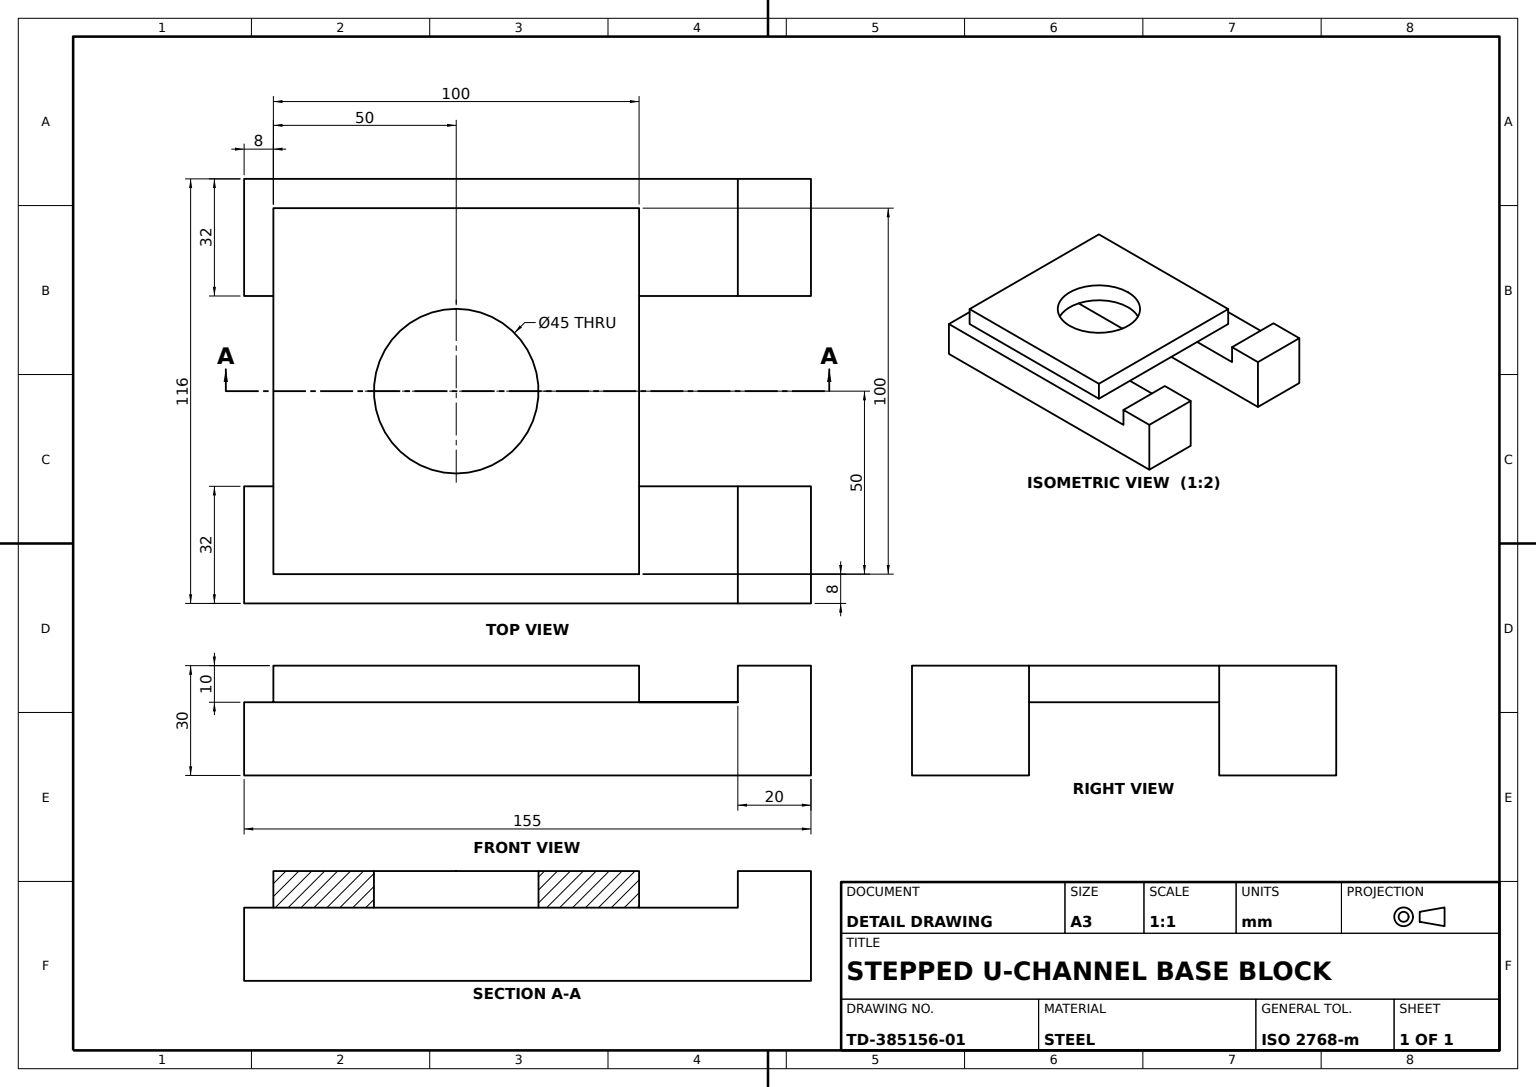
SolidWorks part; units mm, degrees
material "Plain Carbon Steel"
ref_plane "Front Plane" through (0, 0, 0) normal (0, 0, 1) x (1, 0, 0)
ref_plane "Top Plane" through (0, 0, 0) normal (0, 1, 0) x (1, 0, 0)
ref_plane "Right Plane" through (0, 0, 0) normal (1, 0, 0) x (0, 0, -1)
sketch "Base Plate Sketch" plane through (0, 0, 0) normal (0, 1, 0) x (1, 0, 0)
  line L1 (-50, -50) -> (50, -50)
  line L2 (-50, -50) -> (-50, 50)
  line L3 (-50, 50) -> (50, 50)
  line L4 (50, -50) -> (50, 50)
  line L5 (-50, -50) -> (50, 50) construction
  line L6 (-50, 50) -> (50, -50) construction
  circle A0 centre (0, 0) radius 22.5
  point P0 (0, 0)
  dimension "D3" = 45
  dimension "D1" = 100
  dimension "D2" = 100
extrude "Base Plate 100x100 Bore Ø45" add sketch "Base Plate Sketch" along normal blind 10
sketch "Side Rails Sketch" plane through (0, 0, 0) normal (0, -1, 0) x (1, 0, 0)
  line L0 (-50, 50) -> (50, 50) construction
  line L1 (-58, 58) -> (97, 58)
  line L2 (-58, 58) -> (-58, 26)
  line L3 (-58, 26) -> (97, 26)
  line L4 (97, 58) -> (97, 26)
  line L5 (-50, -50) -> (-50, 50) construction
  line L7 (97, -58) -> (97, -26)
  line L8 (-58, -26) -> (97, -26)
  line L9 (-58, -58) -> (-58, -26)
  line L10 (-58, -58) -> (97, -58)
  dimension "D1" = 8
  dimension "D2" = 32
  dimension "D3" = 8
  dimension "D4" = 155
  dimension "D5" = 76
extrude "Side Rails" add sketch "Side Rails Sketch" along normal blind 20 contours L3 L4 L1 L2
sketch "End Blocks Sketch" plane through (0, 0, 0) normal (0, 1, 0) x (1, 0, 0)
  line L0 (97, 26) -> (50, 26) construction
  line L1 (97, 58) -> (77, 58)
  line L2 (97, 58) -> (97, 26)
  line L3 (97, 26) -> (77, 26)
  line L4 (77, 58) -> (77, 26)
  line L5 (97, -58) -> (-58, -58) construction
  line L6 (97, -26) -> (77, -26)
  line L7 (97, -26) -> (97, -58)
  line L8 (97, -58) -> (77, -58)
  line L9 (77, -26) -> (77, -58)
  dimension "D1" = 20
  dimension "D2" = 20
extrude "End Blocks 20x20" add sketch "End Blocks Sketch" along normal blind 10
